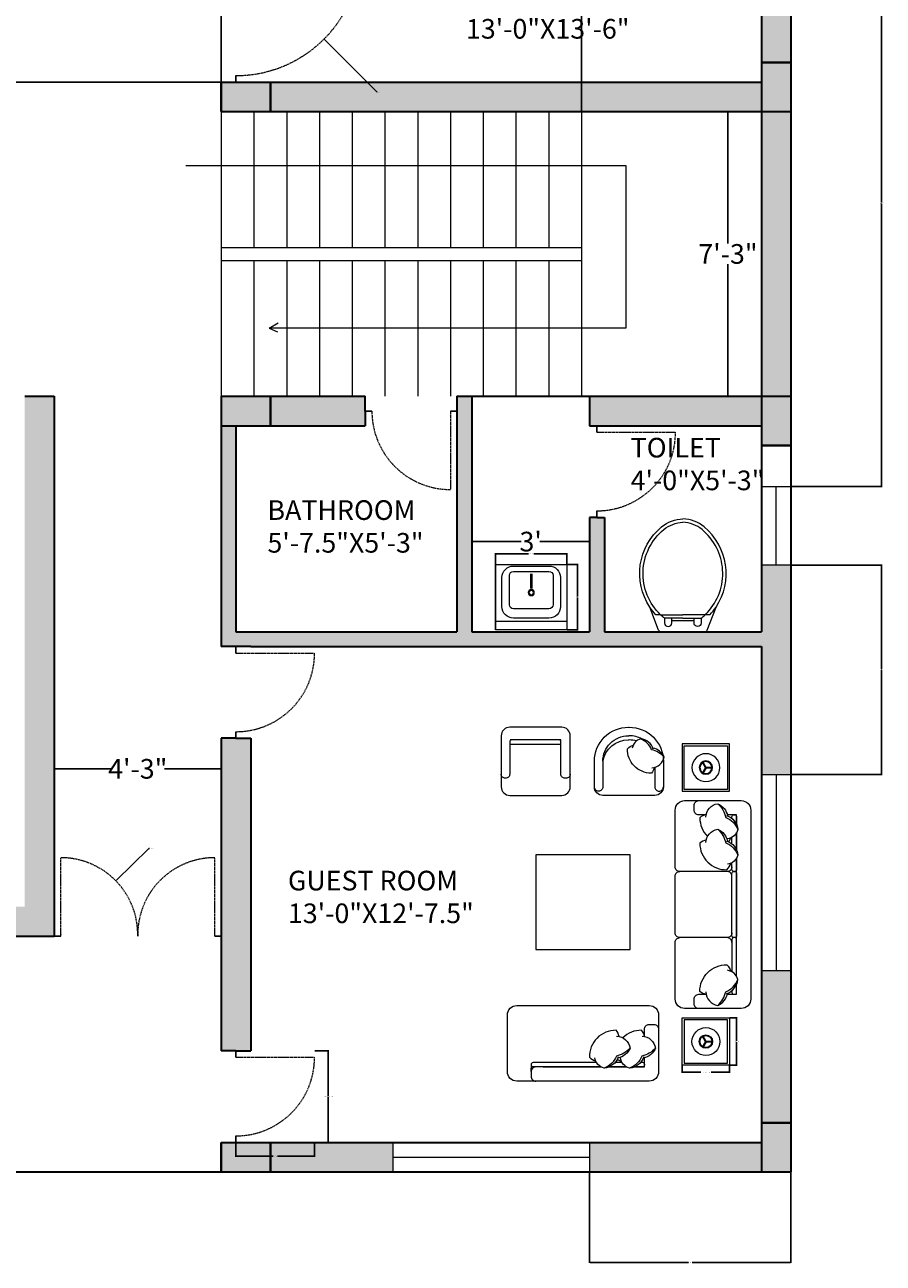
# Model space of a CAD drawing. Units: inches. Extents: x -10 to 455, y -513 to 57.
# Tile 2 of 4: x 193 to 455, y -513 to -134. Entities that reach past the tile are written whole.
import ezdxf

# ---------------------------------------------------------------- set-up
doc = ezdxf.new("R2010")
doc.units = ezdxf.units.IN
doc.header["$MEASUREMENT"] = 0
doc.linetypes.add('DASHED2', pattern=[0.375, 0.25, -0.125])
for name, color, linetype, lineweight in [('A-ANNO-DIMS', 2, 'Continuous', 18), ('A-AREA-IDEN', 7, 'Continuous', 18), ('A-COLS', 7, 'Continuous', 40), ('A-COLS-PATT', 1, 'Continuous', 13), ('A-DOOR', 40, 'DASHED2', 18), ('A-DOOR-FRAM', 7, 'Continuous', 25), ('A-FLOR-FIXT', 9, 'Continuous', 18), ('A-FLOR-STRS', 7, 'Continuous', 18), ('A-FURN', 8, 'Continuous', 13), ('A-GLAZ', 222, 'Continuous', 18), ('A-WALL', 7, 'Continuous', 35), ('A-WALL-PATT', 152, 'Continuous', 13)]:
    doc.layers.add(name, color=color, linetype=linetype, lineweight=lineweight)
doc.styles.get("Standard").update_dxf_attribs({"font": 'arial.ttf'})
doc.dimstyles.get("Standard").update_dxf_attribs({"dimtxt": 0.18, "dimasz": 0.18, "dimexe": 0.18, "dimexo": 0.0625, "dimgap": 0.09, "dimtad": 0, "dimtih": 1, "dimtoh": 1, "dimdec": 0, "dimzin": 0, "dimdsep": 46, "dimlunit": 3, "dimtxsty": 'Standard', "dimcen": 0.09, "dimadec": 0, "dimazin": 0, "dimtfac": 1, "dimtdec": 0, "dimtofl": 0, "dimtmove": 0, "dimatfit": 3, "dimfxl": 1, "dimtolj": 1, "dimtzin": 0, "dimarcsym": 0})

# ---------------------------------------------------------------- blocks, each defined once
blk = doc.blocks.new('*D3')
at = {"layer": 'A-ANNO-DIMS', "color": 0, "lineweight": -2, "transparency": 16777216}
for p, q in [((202.25, -359.95), (202.25, -361.87)), ((202.43, -361.69), (219.56, -361.69)), ((253.07, -361.69), (235.93, -361.69)), ((253.25, -359.95), (253.25, -361.87))]:
    blk.add_line(p, q, dxfattribs=at)
at = {"layer": 'A-ANNO-DIMS', "color": 0, "transparency": 16777216}
for points in [[(202.43, -361.66), (202.43, -361.72), (202.25, -361.69)], [(253.07, -361.66), (253.07, -361.72), (253.25, -361.69)]]:
    blk.add_solid(points, dxfattribs=at)
at = {"layer": 'Defpoints', "color": 0, "transparency": 16777216}
for p in [(202.25, -359.88), (202.25, -361.69), (253.25, -359.88)]:
    blk.add_point(p, dxfattribs=at)
at = {"layer": 'A-ANNO-DIMS', "color": 0, "transparency": 16777216, "insert": (227.75, -361.69), "char_height": 6, "attachment_point": 5}
blk.add_mtext('\\A1;4\'-3"', dxfattribs=at)
blk = doc.blocks.new('*D5')
at = {"layer": 'A-ANNO-DIMS', "color": 0, "lineweight": -2, "transparency": 16777216}
for p, q in [((406.12, -160.85), (408.18, -160.85)), ((408, -161.03), (408, -201.19)), ((408, -247.67), (408, -207.51)), ((406.12, -247.85), (408.18, -247.85))]:
    blk.add_line(p, q, dxfattribs=at)
at = {"layer": 'A-ANNO-DIMS', "color": 0, "transparency": 16777216}
for points in [[(407.97, -161.03), (408.03, -161.03), (408, -160.85)], [(407.97, -247.67), (408.03, -247.67), (408, -247.85)]]:
    blk.add_solid(points, dxfattribs=at)
at = {"layer": 'Defpoints', "color": 0, "transparency": 16777216}
for p in [(406.06, -160.85), (406.06, -247.85), (408, -247.85)]:
    blk.add_point(p, dxfattribs=at)
at = {"layer": 'A-ANNO-DIMS', "color": 0, "transparency": 16777216, "insert": (408, -204.35), "char_height": 6, "attachment_point": 5}
blk.add_mtext('\\A1;7\'-3"', dxfattribs=at)
blk = doc.blocks.new('*D6')
at = {"layer": 'A-ANNO-DIMS', "color": 0, "lineweight": -2, "transparency": 16777216}
for p, q in [((329.75, -291.29), (329.75, -292.44)), ((365.75, -291.29), (365.75, -292.44)), ((329.93, -292.26), (344.9, -292.26)), ((365.57, -292.26), (350.59, -292.26))]:
    blk.add_line(p, q, dxfattribs=at)
at = {"layer": 'A-ANNO-DIMS', "color": 0, "transparency": 16777216}
for points in [[(329.93, -292.23), (329.93, -292.29), (329.75, -292.26)], [(365.57, -292.23), (365.57, -292.29), (365.75, -292.26)]]:
    blk.add_solid(points, dxfattribs=at)
at = {"layer": 'Defpoints', "color": 0, "transparency": 16777216}
for p in [(329.75, -291.23), (365.75, -291.23), (365.75, -292.26)]:
    blk.add_point(p, dxfattribs=at)
at = {"layer": 'A-ANNO-DIMS', "color": 0, "transparency": 16777216, "insert": (347.75, -292.26), "char_height": 6, "attachment_point": 5}
blk.add_mtext("\\A1;3'", dxfattribs=at)
blk = doc.blocks.new('М14 600х655')
for p, q in [((-655, 600), (-655, 0)), ((-655, 600), (-655, 0)), ((-655, 0), (-655, 600)), ((0, 600), (-655, 600)), ((0, 0), (0, 600)), ((0, 525), (-655, 525)), ((-165, 494), (-490, 494)), ((-596, 388), (-596, 121)), ((-528, 370), (-528, 103)), ((-165, 408), (-490, 408)), ((-127, 103), (-127, 370)), ((-59, 121), (-59, 388)), ((-334, 87), (-334, 220)), ((-321, 87), (-321, 220)), ((-655, 0), (-655, 0)), ((-655, 0), (-655, 0)), ((-655, 0), (0, 0)), ((-655, 0), (0, 0)), ((-490, 65), (-165, 65)), ((-490, 15), (-165, 15))]:
    blk.add_line(p, q)
for radius in [27.6, 19.3]:
    blk.add_circle((-327, 259), radius)
for centre, radius, start, end in [((-490, 388), 106, 90, 180), ((-165, 388), 106, 0, 90), ((-490, 370), 38.2, 90, 180), ((-165, 370), 38.2, 0, 90), ((-490, 121), 106, 180, 270), ((-165, 121), 106, 270, 0), ((-490, 103), 38.2, 180, 270), ((-165, 103), 38.2, 270, 0)]:
    blk.add_arc(centre, radius, start, end)
blk = doc.blocks.new('WIN-60IN')
for p, q in [((0, 9), (60, 9)), ((0, 0), (0, 9)), ((60, 9), (60, 0)), ((0, 4.5), (60, 4.5)), ((60, 0), (0, 0))]:
    blk.add_line(p, q)
blk = doc.blocks.new('WIN-24IN')
for p, q in [((0, 9), (24, 9)), ((0, 0), (0, 9)), ((24, 9), (24, 0)), ((0, 4.5), (24, 4.5)), ((24, 0), (0, 0))]:
    blk.add_line(p, q)
blk = doc.blocks.new('DOOR-SINGLE-24IN')
for p, q in [((0, 28), (0, 26)), ((0, 26), (24, 26)), ((0, 0), (0, 2))]:
    blk.add_line(p, q)
blk.add_arc((0, 26), 24, 270, 0)
blk = doc.blocks.new('TABLE-END-WITH-LAMP')
for p, q in [((7.14, 7.17), (6.12, 8.93)), ((7.3, 7.26), (6.28, 9.03)), ((7.14, 7.26), (6.12, 5.5)), ((7.3, 7.17), (6.28, 5.41)), ((7.22, 7.31), (9.25, 7.31)), ((7.22, 7.13), (9.25, 7.13))]:
    blk.add_line(p, q)
at = {"ltscale": 0.03}
blk.add_lwpolyline([(0, 0), (0, 14.43), (14.43, 14.43), (14.43, 0)], close=True, dxfattribs=at)
blk.add_lwpolyline([(0.58, 13.86), (0.58, 0.58), (13.86, 0.58), (13.86, 13.86)], close=True)
for radius in [4.26, 2.04, 1.83]:
    blk.add_circle((7.22, 7.22), radius)
blk = doc.blocks.new('*D16')
at = {"layer": 'A-ANNO-DIMS', "color": 0, "lineweight": -2, "transparency": 16777216}
for p, q in [((281.81, -447.85), (286.13, -447.85)), ((285.95, -448.03), (285.95, -461.67)), ((285.95, -475.67), (285.95, -462.03)), ((281.81, -475.85), (286.13, -475.85))]:
    blk.add_line(p, q, dxfattribs=at)
at = {"layer": 'A-ANNO-DIMS', "color": 0, "transparency": 16777216}
for points in [[(285.92, -448.03), (285.98, -448.03), (285.95, -447.85)], [(285.92, -475.67), (285.98, -475.67), (285.95, -475.85)]]:
    blk.add_solid(points, dxfattribs=at)
at = {"layer": 'Defpoints', "color": 0, "transparency": 16777216}
for p in [(281.75, -447.85), (285.95, -447.85), (281.75, -475.85)]:
    blk.add_point(p, dxfattribs=at)
at = {"layer": 'A-ANNO-DIMS', "color": 0, "transparency": 16777216, "insert": (285.95, -461.85), "char_height": 0.18, "attachment_point": 5}
blk.add_mtext('\\A1;SINGLE DOOR 2\'-4" TYP.', dxfattribs=at)
blk = doc.blocks.new('*D17')
at = {"layer": 'A-ANNO-DIMS', "color": 0, "lineweight": -2, "transparency": 16777216}
for p, q in [((257.75, -475.91), (257.75, -480.23)), ((281.75, -475.91), (281.75, -480.23)), ((257.93, -480.05), (269.11, -480.05)), ((281.57, -480.05), (270.39, -480.05))]:
    blk.add_line(p, q, dxfattribs=at)
at = {"layer": 'A-ANNO-DIMS', "color": 0, "transparency": 16777216}
for points in [[(257.93, -480.02), (257.93, -480.08), (257.75, -480.05)], [(281.57, -480.02), (281.57, -480.08), (281.75, -480.05)]]:
    blk.add_solid(points, dxfattribs=at)
at = {"layer": 'Defpoints', "color": 0, "transparency": 16777216}
for p in [(257.75, -475.85), (281.75, -475.85), (281.75, -480.05)]:
    blk.add_point(p, dxfattribs=at)
at = {"layer": 'A-ANNO-DIMS', "color": 0, "transparency": 16777216, "insert": (269.75, -480.05), "char_height": 0.18, "attachment_point": 5}
blk.add_mtext('\\A1;2\'-0" TYP.', dxfattribs=at)
blk = doc.blocks.new('*D20')
at = {"layer": 'A-ANNO-DIMS', "color": 0, "lineweight": -2, "transparency": 16777216}
for p, q in [((337.03, -299.16), (337.03, -295.77)), ((337.21, -295.95), (347.11, -295.95)), ((358.64, -295.95), (348.73, -295.95)), ((358.82, -299.16), (358.82, -295.77))]:
    blk.add_line(p, q, dxfattribs=at)
at = {"layer": 'A-ANNO-DIMS', "color": 0, "transparency": 16777216}
for points in [[(337.21, -295.92), (337.21, -295.98), (337.03, -295.95)], [(358.64, -295.92), (358.64, -295.98), (358.82, -295.95)]]:
    blk.add_solid(points, dxfattribs=at)
at = {"layer": 'Defpoints', "color": 0, "transparency": 16777216}
for p in [(358.82, -295.95), (337.03, -299.22), (358.82, -299.22)]:
    blk.add_point(p, dxfattribs=at)
at = {"layer": 'A-ANNO-DIMS', "color": 0, "transparency": 16777216, "insert": (347.92, -295.95), "char_height": 0.18, "attachment_point": 5}
blk.add_mtext('\\A1;BASIN 1\'-10"', dxfattribs=at)
blk = doc.blocks.new('*D21')
at = {"layer": 'A-ANNO-DIMS', "color": 0, "lineweight": -2, "transparency": 16777216}
for p, q in [((358.88, -299.22), (362.26, -299.22)), ((362.08, -299.4), (362.08, -309.02)), ((362.08, -319), (362.08, -309.38)), ((358.88, -319.18), (362.26, -319.18))]:
    blk.add_line(p, q, dxfattribs=at)
at = {"layer": 'A-ANNO-DIMS', "color": 0, "transparency": 16777216}
for points in [[(362.05, -299.4), (362.11, -299.4), (362.08, -299.22)], [(362.05, -319), (362.11, -319), (362.08, -319.18)]]:
    blk.add_solid(points, dxfattribs=at)
at = {"layer": 'Defpoints', "color": 0, "transparency": 16777216}
for p in [(358.82, -299.22), (358.82, -319.18), (362.08, -319.18)]:
    blk.add_point(p, dxfattribs=at)
at = {"layer": 'A-ANNO-DIMS', "color": 0, "transparency": 16777216, "insert": (362.08, -309.2), "char_height": 0.18, "attachment_point": 5}
blk.add_mtext('\\A1;1\'-8"', dxfattribs=at)
blk = doc.blocks.new('*D24')
at = {"layer": 'A-ANNO-DIMS', "color": 0, "lineweight": -2, "transparency": 16777216}
for p, q in [((394.05, -452.31), (394.05, -454.6)), ((408.48, -452.31), (408.48, -454.6)), ((394.23, -454.42), (399.69, -454.42)), ((408.3, -454.42), (402.84, -454.42))]:
    blk.add_line(p, q, dxfattribs=at)
at = {"layer": 'A-ANNO-DIMS', "color": 0, "transparency": 16777216}
for points in [[(394.23, -454.39), (394.23, -454.45), (394.05, -454.42)], [(408.3, -454.39), (408.3, -454.45), (408.48, -454.42)]]:
    blk.add_solid(points, dxfattribs=at)
at = {"layer": 'Defpoints', "color": 0, "transparency": 16777216}
for p in [(394.05, -452.25), (408.48, -452.25), (408.48, -454.42)]:
    blk.add_point(p, dxfattribs=at)
at = {"layer": 'A-ANNO-DIMS', "color": 0, "transparency": 16777216, "insert": (401.26, -454.42), "char_height": 0.18, "attachment_point": 5}
blk.add_mtext('\\A1;END TABLE 1\'-2 1/2" TYP.', dxfattribs=at)
blk = doc.blocks.new('*D25')
at = {"layer": 'A-ANNO-DIMS', "color": 0, "lineweight": -2, "transparency": 16777216}
for p, q in [((408.54, -437.82), (410.83, -437.82)), ((410.65, -438), (410.65, -444.85)), ((410.65, -452.07), (410.65, -445.22)), ((408.54, -452.25), (410.83, -452.25))]:
    blk.add_line(p, q, dxfattribs=at)
at = {"layer": 'A-ANNO-DIMS', "color": 0, "transparency": 16777216}
for points in [[(410.62, -438), (410.68, -438), (410.65, -437.82)], [(410.62, -452.07), (410.68, -452.07), (410.65, -452.25)]]:
    blk.add_solid(points, dxfattribs=at)
at = {"layer": 'Defpoints', "color": 0, "transparency": 16777216}
for p in [(408.48, -437.82), (410.65, -437.82), (408.48, -452.25)]:
    blk.add_point(p, dxfattribs=at)
at = {"layer": 'A-ANNO-DIMS', "color": 0, "transparency": 16777216, "insert": (410.65, -445.03), "char_height": 0.18, "attachment_point": 5}
blk.add_mtext('\\A1;1\'-2 1/2" TYP.', dxfattribs=at)
blk = doc.blocks.new('*D38')
at = {"layer": 'A-ANNO-DIMS', "color": 0, "lineweight": -2, "transparency": 16777216}
for p, q in [((427.31, -102.17), (455.08, -102.17)), ((454.9, -102.35), (454.9, -188.62)), ((454.9, -275.26), (454.9, -188.98)), ((427.31, -275.44), (455.08, -275.44))]:
    blk.add_line(p, q, dxfattribs=at)
at = {"layer": 'A-ANNO-DIMS', "color": 0, "transparency": 16777216}
for points in [[(454.87, -102.35), (454.93, -102.35), (454.9, -102.17)], [(454.87, -275.26), (454.93, -275.26), (454.9, -275.44)]]:
    blk.add_solid(points, dxfattribs=at)
at = {"layer": 'Defpoints', "color": 0, "transparency": 16777216}
for p in [(427.25, -102.17), (427.25, -275.44), (454.9, -275.44)]:
    blk.add_point(p, dxfattribs=at)
at = {"layer": 'A-ANNO-DIMS', "color": 0, "transparency": 16777216, "insert": (454.9, -188.8), "char_height": 0.18, "attachment_point": 5}
blk.add_mtext('\\A1;14\'-5 1/2"', dxfattribs=at)
blk = doc.blocks.new('*D39')
at = {"layer": 'A-ANNO-DIMS', "color": 0, "lineweight": -2, "transparency": 16777216}
for p, q in [((427.31, -299.44), (455.08, -299.44)), ((454.9, -299.62), (454.9, -331.23)), ((454.9, -363.21), (454.9, -331.59)), ((427.31, -363.39), (455.08, -363.39))]:
    blk.add_line(p, q, dxfattribs=at)
at = {"layer": 'A-ANNO-DIMS', "color": 0, "transparency": 16777216}
for points in [[(454.87, -299.62), (454.93, -299.62), (454.9, -299.44)], [(454.87, -363.21), (454.93, -363.21), (454.9, -363.39)]]:
    blk.add_solid(points, dxfattribs=at)
at = {"layer": 'Defpoints', "color": 0, "transparency": 16777216}
for p in [(427.25, -299.44), (427.25, -363.39), (454.9, -363.39)]:
    blk.add_point(p, dxfattribs=at)
at = {"layer": 'A-ANNO-DIMS', "color": 0, "transparency": 16777216, "insert": (454.9, -331.41), "char_height": 0.18, "attachment_point": 5}
blk.add_mtext('\\A1;5\'-4"', dxfattribs=at)
blk = doc.blocks.new('*D40')
at = {"layer": 'A-ANNO-DIMS', "color": 0, "lineweight": -2, "transparency": 16777216}
for p, q in [((365.75, -484.91), (365.75, -512.68)), ((427.25, -484.91), (427.25, -512.68)), ((365.93, -512.5), (395.96, -512.5)), ((427.07, -512.5), (397.04, -512.5))]:
    blk.add_line(p, q, dxfattribs=at)
at = {"layer": 'A-ANNO-DIMS', "color": 0, "transparency": 16777216}
for points in [[(365.93, -512.47), (365.93, -512.53), (365.75, -512.5)], [(427.07, -512.47), (427.07, -512.53), (427.25, -512.5)]]:
    blk.add_solid(points, dxfattribs=at)
at = {"layer": 'Defpoints', "color": 0, "transparency": 16777216}
for p in [(365.75, -484.85), (427.25, -484.85), (427.25, -512.5)]:
    blk.add_point(p, dxfattribs=at)
at = {"layer": 'A-ANNO-DIMS', "color": 0, "transparency": 16777216, "insert": (396.5, -512.5), "char_height": 0.18, "attachment_point": 5}
blk.add_mtext('\\A1;5\'-1 1/2"', dxfattribs=at)
blk = doc.blocks.new('*D41')
at = {"layer": 'A-ANNO-DIMS', "color": 0, "lineweight": -2, "transparency": 16777216}
for p, q in [((253.25, -160.79), (253.25, 46.98)), ((253.43, 46.8), (307.92, 46.8)), ((363.07, 46.8), (308.58, 46.8)), ((363.25, -160.79), (363.25, 46.98))]:
    blk.add_line(p, q, dxfattribs=at)
at = {"layer": 'A-ANNO-DIMS', "color": 0, "transparency": 16777216}
for points in [[(253.43, 46.83), (253.43, 46.77), (253.25, 46.8)], [(363.07, 46.83), (363.07, 46.77), (363.25, 46.8)]]:
    blk.add_solid(points, dxfattribs=at)
at = {"layer": 'Defpoints', "color": 0, "transparency": 16777216}
for p in [(363.25, 46.8), (253.25, -160.85), (363.25, -160.85)]:
    blk.add_point(p, dxfattribs=at)
at = {"layer": 'A-ANNO-DIMS', "color": 0, "transparency": 16777216, "insert": (308.25, 46.8), "char_height": 0.18, "attachment_point": 5}
blk.add_mtext('\\A1;9\'-2"', dxfattribs=at)
blk = doc.blocks.new('*D43')
at = {"layer": 'A-ANNO-DIMS', "color": 0, "lineweight": -2, "transparency": 16777216}
for p, q in [((253.18, -109.85), (12.42, -109.85)), ((12.6, -110.03), (12.6, -130.67)), ((12.6, -151.67), (12.6, -131.03)), ((253.18, -151.85), (12.42, -151.85))]:
    blk.add_line(p, q, dxfattribs=at)
at = {"layer": 'A-ANNO-DIMS', "color": 0, "transparency": 16777216}
for points in [[(12.57, -110.03), (12.63, -110.03), (12.6, -109.85)], [(12.57, -151.67), (12.63, -151.67), (12.6, -151.85)]]:
    blk.add_solid(points, dxfattribs=at)
at = {"layer": 'Defpoints', "color": 0, "transparency": 16777216}
for p in [(253.25, -109.85), (12.6, -151.85), (253.25, -151.85)]:
    blk.add_point(p, dxfattribs=at)
at = {"layer": 'A-ANNO-DIMS', "color": 0, "transparency": 16777216, "insert": (12.6, -130.85), "char_height": 0.18, "attachment_point": 5}
blk.add_mtext('\\A1;3\'-6"', dxfattribs=at)
blk = doc.blocks.new('*D45')
at = {"layer": 'A-ANNO-DIMS', "color": 0, "lineweight": -2, "transparency": 16777216}
for p, q in [((257.66, -111.85), (257.84, -111.85)), ((257.75, -111.94), (257.75, -111.76)), ((300.74, -154.84), (284.74, -138.85)), ((300.92, -154.84), (300.74, -154.84))]:
    blk.add_line(p, q, dxfattribs=at)
at = {"layer": 'A-ANNO-DIMS', "color": 0, "transparency": 16777216}
blk.add_solid([(284.76, -138.83), (284.72, -138.87), (284.62, -138.72)], dxfattribs=at)
at = {"layer": 'Defpoints', "color": 0, "transparency": 16777216}
for p in [(257.75, -111.85), (284.62, -138.72)]:
    blk.add_point(p, dxfattribs=at)
at = {"layer": 'A-ANNO-DIMS', "color": 0, "transparency": 16777216, "insert": (301.33, -154.84), "char_height": 0.18, "attachment_point": 5}
blk.add_mtext('\\A1;R3\'-2"', dxfattribs=at)
blk = doc.blocks.new('*D46')
at = {"layer": 'A-ANNO-DIMS', "color": 0, "lineweight": -2, "transparency": 16777216}
for p, q in [((231.12, -386.04), (221.17, -395.79)), ((231.3, -386.04), (231.12, -386.04)), ((204.16, -412.36), (204.34, -412.36)), ((204.25, -412.45), (204.25, -412.27))]:
    blk.add_line(p, q, dxfattribs=at)
at = {"layer": 'A-ANNO-DIMS', "color": 0, "transparency": 16777216}
blk.add_solid([(221.15, -395.76), (221.19, -395.81), (221.04, -395.91)], dxfattribs=at)
at = {"layer": 'Defpoints', "color": 0, "transparency": 16777216}
for p in [(221.04, -395.91), (204.25, -412.36)]:
    blk.add_point(p, dxfattribs=at)
at = {"layer": 'A-ANNO-DIMS', "color": 0, "transparency": 16777216, "insert": (232.19, -386.04), "char_height": 0.18, "attachment_point": 5}
blk.add_mtext('\\A1;2X R1\'-11 1/2"', dxfattribs=at)

msp = doc.modelspace()

# ---------------------------------------------------------------- hatches: boundary and pattern name
at = {"layer": 'A-COLS-PATT'}
h = msp.add_hatch(color=256, dxfattribs=at)
h.dxf.hatch_style = 1
h.paths.add_polyline_path([(55.25, 19.15), (40.25, 19.15), (40.25, 10.15), (55.25, 10.15)])
h.paths.add_polyline_path([(262.25, 19.15), (253.25, 19.15), (253.25, 4.15), (262.25, 4.15)])
h.paths.add_polyline_path([(427.25, 19.15), (418.25, 19.15), (418.25, 4.15), (427.25, 4.15)])
h.paths.add_polyline_path([(427.25, -247.85), (418.25, -247.85), (418.25, -262.85), (427.25, -262.85)])
h.paths.add_polyline_path([(268.25, -247.85), (253.25, -247.85), (253.25, -256.85), (268.25, -256.85)])
h.paths.add_polyline_path([(55.25, -247.85), (40.25, -247.85), (40.25, -256.85), (55.25, -256.85)])
h.paths.add_polyline_path([(55.25, -475.85), (49.25, -475.85), (40.25, -475.85), (40.25, -484.85), (55.25, -484.85)])
h.paths.add_polyline_path([(268.25, -475.85), (253.25, -475.85), (253.25, -484.85), (268.25, -484.85)])
h.paths.add_polyline_path([(427.25, -469.85), (418.25, -469.85), (418.25, -484.85), (427.25, -484.85)])
h.paths.add_polyline_path([(55.25, -100.85), (40.25, -100.85), (40.25, -109.85), (55.25, -109.85)])
h = msp.add_hatch(color=256, dxfattribs=at)
h.dxf.hatch_style = 1
h.paths.add_polyline_path([(268.25, -151.85), (253.25, -151.85), (253.25, -160.85), (268.25, -160.85)])
h.paths.add_polyline_path([(427.25, -145.85), (418.25, -145.85), (418.25, -160.85), (427.25, -160.85)])
at = {"layer": 'A-WALL-PATT'}
h = msp.add_hatch(color=256, dxfattribs=at)
h.dxf.hatch_style = 1
h.paths.add_polyline_path([(418.25, -151.85), (268.25, -151.85), (268.25, -160.85), (418.25, -160.85)])
h.paths.add_polyline_path([(165.25, -100.85), (55.25, -100.85), (55.25, -109.85), (165.25, -109.85), (165.25, -105.35)])
h.paths.add_polyline_path([(49.25, -75.35), (40.25, -75.35), (40.25, -100.85), (49.25, -100.85)])
h.paths.add_polyline_path([(49.25, 10.15), (40.25, 10.15), (40.25, -15.35), (49.25, -15.35)])
h.paths.add_polyline_path([(86.75, 19.15), (55.25, 19.15), (55.25, 10.15), (86.75, 10.15)])
h.paths.add_polyline_path([(213.5, 19.15), (146.75, 19.15), (146.75, 10.15), (193.25, 10.15), (193.25, -28.04), (197.75, -28.04), (197.75, 10.15), (213.5, 10.15)])
h.paths.add_polyline_path([(262.25, 4.15), (253.25, 4.15), (253.25, -69.35), (197.75, -69.35), (197.75, -60), (193.25, -60), (193.25, -109.85), (197.75, -109.85), (197.75, -73.85), (253.25, -73.85), (253.25, -109.85), (262.25, -109.85)])
h.paths.add_polyline_path([(310.25, 19.15), (262.25, 19.15), (262.25, 10.15), (310.25, 10.15)])
h.paths.add_polyline_path([(253.25, 19.15), (237.5, 19.15), (237.5, 10.15), (253.25, 10.15)])
h.paths.add_polyline_path([(418.25, 19.15), (370.25, 19.15), (370.25, 10.15), (418.25, 10.15)])
h.paths.add_polyline_path([(427.25, 4.15), (418.25, 4.15), (418.25, -42.17), (427.25, -42.17)])
h.paths.add_polyline_path([(427.25, -102.17), (418.25, -102.17), (418.25, -145.85), (427.25, -145.85)])
h.paths.add_polyline_path([(427.25, -160.85), (418.25, -160.85), (418.25, -247.85), (427.25, -247.85)])
h.paths.add_polyline_path([(418.25, -247.85), (365.75, -247.85), (365.75, -256.85), (418.25, -256.85)], flags=17)
h.paths.add_polyline_path([(297.25, -247.85), (268.25, -247.85), (268.25, -256.85), (297.25, -256.85), (297.25, -252.35)], flags=17)
h.paths.add_polyline_path([(427.25, -299.44), (418.25, -299.44), (418.25, -319.85), (370.25, -319.85), (370.25, -284.85), (368, -284.85), (365.75, -284.85), (365.75, -319.85), (329.75, -319.85), (329.75, -247.85), (325.25, -247.85), (325.25, -319.85), (257.75, -319.85), (257.75, -256.85), (253.25, -256.85), (253.25, -324.35), (262.25, -324.35), (418.25, -324.35), (418.25, -363.39), (427.25, -363.39)])
h.paths.add_polyline_path([(262.25, -352.35), (257.75, -352.35), (253.25, -352.35), (253.25, -447.85), (257.75, -447.85), (262.25, -447.85)])
h.paths.add_polyline_path([(305.75, -475.85), (268.25, -475.85), (268.25, -484.85), (305.75, -484.85)])
h.paths.add_polyline_path([(418.25, -475.85), (365.75, -475.85), (365.75, -484.85), (418.25, -484.85)])
h.paths.add_polyline_path([(427.25, -423.39), (418.25, -423.39), (418.25, -469.85), (427.25, -469.85)])
h.paths.add_polyline_path([(202.25, -247.85), (193.25, -247.85), (193.25, -403.85), (49.25, -403.85), (49.25, -360.35), (40.25, -360.35), (40.25, -412.85), (202.25, -412.85)])
h.paths.add_polyline_path([(165.25, -247.85), (55.25, -247.85), (55.25, -256.85), (165.25, -256.85), (165.25, -252.35)], flags=17)
h.paths.add_polyline_path([(49.25, -225.11), (40.25, -225.11), (40.25, -247.85), (49.25, -247.85)])
h.paths.add_polyline_path([(49.25, -256.85), (40.25, -256.85), (40.25, -300.35), (49.25, -300.35)], flags=17)
h.paths.add_polyline_path([(49.25, -137.85), (44.75, -137.85), (40.25, -137.85), (40.25, -165.11), (49.25, -165.11)])

# ---------------------------------------------------------------- linework, layer by layer
at = {"layer": 'A-COLS'}
for p, q in [((418.25, -145.85), (427.25, -145.85)), ((253.25, -151.85), (253.25, -160.85)), ((268.25, -151.85), (268.25, -160.85)), ((268.25, -256.85), (268.25, -247.85)), ((418.25, -262.85), (427.25, -262.85)), ((418.25, -469.85), (427.25, -469.85)), ((253.25, -475.85), (253.25, -484.85)), ((268.25, -475.85), (268.25, -484.85))]:
    msp.add_line(p, q, dxfattribs=at)
at = {"layer": 'A-DOOR'}
for p, q in [((257.75, -149.85), (257.75, -151.85)), ((204.25, -412.85), (204.25, -388.85)), ((251.25, -412.85), (251.25, -388.85)), ((202.25, -412.85), (204.25, -412.85)), ((253.25, -412.85), (251.25, -412.85))]:
    msp.add_line(p, q, dxfattribs=at)
for centre, radius, start, end in [((257.75, -111.85), 38, 270, 0), ((204.25, -412.36), 23.51, 358.7938, 90), ((251.25, -412.36), 23.51, 90, 181.2062)]:
    msp.add_arc(centre, radius, start, end, dxfattribs=at)
at = {"layer": 'A-DOOR-FRAM'}
for p, q in [((257.75, -151.85), (257.75, -149.85)), ((299.25, -252.35), (297.25, -252.35)), ((325.25, -252.35), (323.25, -252.35)), ((368, -256.85), (368, -258.85)), ((368, -282.85), (368, -284.85)), ((257.75, -324.35), (257.75, -326.35)), ((257.75, -350.35), (257.75, -352.35)), ((202.25, -412.85), (204.25, -412.85)), ((253.25, -412.85), (251.25, -412.85)), ((257.75, -449.85), (257.75, -447.85)), ((257.75, -475.85), (257.75, -473.85))]:
    msp.add_line(p, q, dxfattribs=at)
at = {"layer": 'A-FLOR-FIXT'}
for p, q in [((387.45, -314.62), (386, -314.62)), ((387.45, -314.62), (394.25, -314.62)), ((401.04, -314.62), (394.25, -314.62)), ((402.49, -314.62), (401.04, -314.62))]:
    msp.add_line(p, q, dxfattribs=at)
for points in [[(384.13, -312.25, -0.383919), (387.75, -287.78, -0.163732), (394.25, -285.29, -0.359733)], [(387.45, -314.62, -0.448546), (388.41, -288.58, -0.162618), (394.25, -286.33, -0.470877)], [(404.36, -312.25, 0.383919), (400.74, -287.78, 0.163732), (394.25, -285.29, 0.359733)], [(401.74, -313.91, 0.431639), (400.08, -288.58, 0.162618), (394.25, -286.33, 0.470877)], [(386, -314.62, -0.040937), (384.13, -312.25, -0.163732)], [(394.25, -319.85), (387.65, -319.85, -0.31031), (386.84, -319.3), (384.13, -312.25, -0.209071)], [(394.25, -319.85), (400.84, -319.85, 0.31031), (401.65, -319.3), (404.36, -312.25, 0.209071)], [(401.04, -314.62, 0.014165), (401.74, -313.91, 0.162618)], [(402.49, -314.62, 0.040937), (404.36, -312.25, 0.163732)], [(388.64, -315.66, -0.022712), (387.45, -314.62, -0.162618)], [(394.25, -315.66), (388.64, -315.66, -0.476108)], [(388.64, -315.66), (388.64, -317.11, 1), (390.84, -317.11), (390.84, -316.36)], [(394.25, -315.66), (399.85, -315.66, 0.022712)], [(399.85, -315.66), (399.85, -317.11, -1), (397.65, -317.11), (397.65, -316.36)], [(399.85, -315.66, 0.022712), (401.04, -314.62, 0.162618)]]:
    msp.add_lwpolyline(points, format="xyb", dxfattribs=at)
for points in [[(390.84, -316.36), (390.84, -315.66)], [(390.84, -316.36), (397.65, -316.36)], [(397.65, -316.36), (397.65, -315.66)]]:
    msp.add_lwpolyline(points, dxfattribs=at)
at = {"layer": 'A-FLOR-STRS'}
for p, q in [((253.25, -160.85), (253.25, -247.85)), ((263.25, -160.85), (263.25, -202.35)), ((273.25, -160.85), (273.25, -202.35)), ((283.25, -160.85), (283.25, -202.35)), ((293.25, -160.85), (293.25, -202.35)), ((303.25, -160.85), (303.25, -202.35)), ((313.25, -160.85), (313.25, -202.35)), ((323.25, -160.85), (323.25, -202.35)), ((333.25, -160.85), (333.25, -202.35)), ((343.25, -160.85), (343.25, -202.35)), ((353.25, -160.85), (353.25, -202.35)), ((363.25, -160.85), (363.25, -247.85)), ((242.44, -177.35), (376.77, -177.35)), ((376.77, -177.35), (376.77, -227.04)), ((253.25, -202.35), (363.25, -202.35)), ((253.25, -206.35), (363.25, -206.35)), ((263.25, -206.35), (263.25, -247.85)), ((273.25, -206.35), (273.25, -247.85)), ((283.25, -206.35), (283.25, -247.85)), ((293.25, -206.35), (293.25, -247.85)), ((303.25, -206.35), (303.25, -247.85)), ((313.25, -206.35), (313.25, -247.85)), ((323.25, -206.35), (323.25, -247.85)), ((333.25, -206.35), (333.25, -247.85)), ((343.25, -206.35), (343.25, -247.85)), ((353.25, -206.35), (353.25, -247.85)), ((267.87, -227.04), (270.59, -225.4)), ((376.77, -227.04), (267.87, -227.04)), ((267.87, -227.04), (270.38, -228.11))]:
    msp.add_line(p, q, dxfattribs=at)
at = {"layer": 'A-FURN'}
msp.add_line((347.86, -454.23), (348, -452.07), dxfattribs=at)
at = {"layer": 'A-FURN', "ltscale": 0.03}
for points in [[(341.36, -348.98), (341.36, -348.98, 0.414214), (338.75, -351.58), (338.75, -367.2, 0.414214), (341.36, -369.8), (341.36, -369.8), (357.23, -369.8, 0.414214), (359.84, -367.2), (359.84, -351.58, 0.414214), (357.23, -348.98)], [(394.77, -434.93, -0.414214), (391.88, -432.04), (391.88, -414.72, -0.414214), (393.33, -413.28, -0.414214), (391.88, -411.83), (391.88, -394.51, -0.414214), (393.33, -393.07, -0.414214), (391.88, -391.63), (391.88, -374.31, -0.414214), (394.77, -371.42), (412.09, -371.42, -0.414214), (414.98, -374.31), (414.98, -432.04, -0.414214), (412.09, -434.93)], [(340.64, -436.91, -0.414214), (343.53, -434.02), (343.53, -434.02, 0.317837), (343.53, -434.02, -0.414214), (343.53, -434.02), (343.53, -434.02, 1.186185), (343.53, -434.02, -0.414214), (343.53, -434.02), (383.94, -434.02, -0.414214), (386.83, -436.91), (386.83, -454.23, -0.414214), (383.94, -457.12), (343.53, -457.12, -0.414214), (340.64, -454.23)]]:
    msp.add_lwpolyline(points, format="xyb", close=True, dxfattribs=at)
msp.add_lwpolyline([(377.74, -369.8), (369.8, -369.8, -0.414214), (367.2, -367.2), (367.2, -359.39, -0.414214), (377.61, -348.98), (377.74, -348.98), (377.87, -348.98, -0.414214), (388.28, -359.39), (388.28, -367.2, -0.414214), (385.68, -369.8), (377.74, -369.8)], format="xyb", dxfattribs=at)
at = {"layer": 'A-FURN'}
for points in [[(369.8, -359.39, -0.414214), (377.61, -351.58), (377.74, -351.58)], [(381.74, -352.61, 0.130591), (377.87, -351.58), (377.74, -351.58)], [(341.36, -353.66), (341.36, -363.29, -0.414214), (340.05, -364.59), (340.05, -364.59, -0.414214), (338.75, -363.29)], [(352.07, -352.88), (341.88, -352.88, 0.414214), (341.36, -353.4), (341.36, -353.66, 0.414214), (341.88, -354.18), (350.76, -354.18, 0.414214)], [(350.76, -354.18), (356.45, -354.18, 0.414214), (356.97, -353.66), (356.97, -353.4, 0.414214), (356.45, -352.88)], [(356.45, -352.88), (352.07, -352.88, 0.414214)], [(369.8, -359.39, -0.372719), (377.61, -352.88), (377.74, -352.88)], [(385.42, -361.28, -0.165541), (384.61, -363, -0.425989), (377.3, -355.54, -0.121523), (379.04, -354.51, 7.115464)], [(380.09, -353.16, 0.072384), (377.87, -352.88), (377.74, -352.88)], [(385.21, -355.66, 0.306663), (381.33, -352.56, 0.30633), (378.8, -355.39, -0.872847)], [(388.49, -358.07, 0.14773), (384.69, -355.84, 0.213343), (381.33, -352.56, 0.178662)], [(384.76, -361.35, 0.356772), (388.49, -358.07, 0.249542), (385.11, -355.37, -9.61688)], [(369.8, -359.39), (369.8, -367.2, -0.414214), (368.5, -368.5), (368.5, -368.5, -0.414214), (367.2, -367.2)], [(359.84, -363.29, -0.414214), (358.54, -364.59), (358.28, -364.59, -0.414214), (356.97, -363.29), (356.97, -361.28)], [(385.68, -361.21), (385.68, -367.2, 0.414214), (386.98, -368.5), (386.98, -368.5, 0.414214), (388.28, -367.2)], [(401.34, -375.75), (399.1, -375.75, -0.414214), (397.66, -374.31), (397.66, -372.86, -0.414214), (399.1, -371.42)], [(401.25, -376.47, -0.356772), (404.89, -372.34, -0.249542), (407.89, -376.08)], [(404.89, -372.34, -0.14773), (407.37, -376.56, -0.213343), (411.01, -380.28)], [(401.34, -375.75, 0.165541), (399.43, -376.64, 0.200231), (401.75, -382.37)], [(407.57, -375.97, -0.306663), (411.01, -380.28, -0.30633), (407.86, -383.09)], [(410.65, -378.79), (410.65, -375.75), (407.81, -375.75, -0.414352)], [(409.2, -376.85), (409.2, -376.33, -0.414214), (409.78, -375.75), (410.07, -375.75, -0.414214), (410.65, -376.33)], [(410.65, -376.33), (410.65, -378.79, -0.414469)], [(401.25, -384.25, -0.356772), (404.89, -380.11, -0.249542), (407.89, -383.86)], [(404.89, -380.11, -0.14773), (407.37, -384.33, -0.213343), (411.01, -388.05)], [(410.65, -381.19), (410.65, -386.56, -0.414747)], [(401.34, -383.52, 0.165541), (399.43, -384.41, 0.425989), (407.7, -392.52, 0.121523), (408.84, -390.6)], [(407.57, -383.75, -0.306663), (411.01, -388.05, -0.30633), (407.86, -390.87)], [(408.27, -384.03, 0.071865), (408.84, -382.82)], [(409.2, -384.63), (409.2, -382.64, -0.414599)], [(410.65, -388.96), (410.65, -392.49, -0.414214), (410.07, -393.07), (409.78, -393.07, -0.414214), (409.2, -392.49), (409.2, -390.42, -0.126313)], [(409.2, -391.63, -0.414214), (407.76, -393.07), (393.33, -393.07, -0.41732)], [(409.2, -394.51, 0.414214), (407.76, -393.07)], [(409.2, -411.83, -0.414214), (407.76, -413.28)], [(409.2, -414.72, 0.414214), (407.76, -413.28), (393.33, -413.28, 0.415249)], [(410.65, -425.16), (410.65, -413.86, 0.414214), (410.07, -413.28), (409.78, -413.28, 0.414214), (409.2, -413.86), (409.2, -423.71, 0.412652)], [(401.34, -430.6, -0.165541), (399.43, -429.71, -0.425989), (407.7, -421.6, -0.121523), (408.84, -423.53)], [(407.57, -430.37, 0.306663), (411.01, -426.07, 0.30633), (407.86, -423.26)], [(404.89, -434.01, 0.14773), (407.37, -429.79, 0.213343), (411.01, -426.07)], [(410.65, -430.02), (410.65, -427.56, 0.412535)], [(399.1, -434.93, -0.414214), (397.66, -433.49), (397.66, -432.04, -0.414214), (399.1, -430.6), (401.34, -430.6)], [(401.25, -429.87, 0.356772), (404.89, -434.01, 0.249542), (407.89, -430.26)], [(409.2, -429.5), (409.2, -430.02, 0.414214), (409.78, -430.6), (410.07, -430.6, 0.414214), (410.65, -430.02)], [(374.73, -443.48, 0.165541), (373.83, -441.57, 0.425989), (365.73, -449.84, 0.121523), (367.65, -450.98, -7.115464)], [(382.5, -443.48, 0.165541), (381.61, -441.57, 0.200231), (375.88, -443.89, 0.121523)], [(382.5, -443.48), (382.5, -441.24, -0.414214), (383.94, -439.8), (385.39, -439.8, -0.414214), (386.83, -441.24)], [(374, -443.39, -0.356772), (378.14, -447.03, -0.249542), (374.39, -450.03, 9.61688)], [(381.78, -443.39, -0.356772), (385.91, -447.03, -0.249542), (382.16, -450.03, 9.61688)], [(374.5, -449.71, -0.306663), (370.2, -453.15, -0.30633), (367.38, -450, 0.872847)], [(378.14, -447.03, -0.14773), (373.92, -449.51, -0.213343), (370.2, -453.15, -0.178662)], [(382.28, -449.71, -0.306663), (377.97, -453.15, -0.30633), (375.16, -450, 0.872847)], [(385.91, -447.03, -0.14773), (381.69, -449.51, -0.213343), (377.97, -453.15, -0.178662)], [(379.46, -452.79), (382.5, -452.79), (382.5, -449.95, -0.414214)], [(351.54, -452.79), (349.3, -452.79, 0.414214), (347.86, -454.23), (347.86, -455.67, 0.414214), (349.3, -457.12)], [(369.29, -452.79), (348.58, -452.79, -0.414214), (348, -452.21), (348, -451.92, -0.414214), (348.58, -451.34), (367.83, -451.34, -0.414214)], [(377.06, -452.79), (371.69, -452.79, -0.414214)], [(373.62, -451.34), (375.61, -451.34, -0.414214)], [(374.22, -450.41, 0.071865), (375.43, -450.98, -7.115464)], [(381.92, -452.79), (379.46, -452.79, -0.414214)], [(381.4, -451.34), (381.92, -451.34, -0.414214), (382.5, -451.92), (382.5, -452.21, -0.414214), (381.92, -452.79)]]:
    msp.add_lwpolyline(points, format="xyb", dxfattribs=at)
for points in [[(352.07, -352.88), (341.49, -352.88)], [(356.97, -361.28), (356.97, -352.88), (352.07, -352.88)], [(410.65, -386.56), (410.65, -381.19)], [(410.65, -425.16), (410.65, -388.96)], [(407.81, -430.6), (410.65, -430.6), (410.65, -427.56)], [(351.54, -452.79), (369.29, -452.79)], [(371.69, -452.79), (377.06, -452.79)]]:
    msp.add_lwpolyline(points, dxfattribs=at)
at = {"layer": 'A-FURN', "ltscale": 0.03}
msp.add_lwpolyline([(349.3, -388.02), (349.3, -416.89), (378.17, -416.89), (378.17, -388.02)], close=True, dxfattribs=at)
at = {"layer": 'A-FURN'}
msp.add_lwpolyline([(410.65, -393.65), (410.65, -412.7, -0.414214), (410.07, -413.28), (409.78, -413.28, -0.414214), (409.2, -412.7), (409.2, -393.65, -0.414214), (409.78, -393.07), (410.07, -393.07, -0.414214)], format="xyb", close=True, dxfattribs=at)
at = {"layer": 'A-WALL'}
for p, q in [((418.25, 19.15), (418.25, -319.85)), ((427.25, 19.15), (427.25, -484.85)), ((253.25, -151.85), (418.25, -151.85)), ((253.25, -160.85), (427.25, -160.85)), ((193.25, -247.85), (202.25, -247.85)), ((202.25, -247.85), (202.25, -412.85)), ((253.25, -247.85), (297.25, -247.85)), ((253.25, -247.85), (253.25, -324.35)), ((297.25, -252.35), (297.25, -247.85)), ((325.25, -247.85), (325.25, -319.85)), ((325.25, -247.85), (427.25, -247.85)), ((329.75, -247.85), (329.75, -319.85)), ((365.75, -247.85), (365.75, -256.85)), ((297.25, -252.35), (297.25, -256.85)), ((253.25, -256.85), (297.25, -256.85)), ((257.75, -256.85), (257.75, -319.85)), ((365.75, -256.85), (418.25, -256.85)), ((368, -284.85), (365.75, -284.85)), ((365.75, -284.85), (365.75, -319.85)), ((368, -284.85), (370.25, -284.85)), ((370.25, -284.85), (370.25, -319.85)), ((257.75, -319.85), (325.25, -319.85)), ((329.75, -319.85), (365.75, -319.85)), ((370.25, -319.85), (418.25, -319.85)), ((262.25, -324.35), (253.25, -324.35)), ((262.25, -324.35), (418.25, -324.35)), ((418.25, -324.35), (418.25, -484.85)), ((257.75, -352.35), (253.25, -352.35)), ((253.25, -352.35), (253.25, -447.85)), ((257.75, -352.35), (262.25, -352.35)), ((262.25, -352.35), (262.25, -447.85)), ((40.25, -412.85), (202.25, -412.85)), ((257.75, -447.85), (253.25, -447.85)), ((257.75, -447.85), (262.25, -447.85)), ((253.25, -475.85), (418.25, -475.85)), ((40.25, -484.85), (427.25, -484.85))]:
    msp.add_line(p, q, dxfattribs=at)

# ---------------------------------------------------------------- block references
at = {"layer": 'A-DOOR', "rotation": 270}
msp.add_blockref('DOOR-SINGLE-24IN', (297.25, -252.35), dxfattribs=at)
at = {"layer": 'A-DOOR'}
for p in [(368, -284.85), (257.75, -352.35), (257.75, -475.85)]:
    msp.add_blockref('DOOR-SINGLE-24IN', p, dxfattribs=at)
at = {"layer": 'A-FLOR-FIXT', "xscale": -0.033266506394089, "yscale": 0.033266506394089, "zscale": 0.033266506394089, "rotation": 180}
msp.add_blockref('М14 600х655', (358.82, -299.22), dxfattribs=at)
at = {"layer": 'A-FURN', "extrusion": (0, 0, -1), "zscale": -1, "rotation": 180}
msp.add_blockref('TABLE-END-WITH-LAMP', (-394.05, -354.1), dxfattribs=at)
at = {"layer": 'A-FURN'}
msp.add_blockref('TABLE-END-WITH-LAMP', (394.05, -452.25), dxfattribs=at)
at = {"layer": 'A-GLAZ'}
for name, p, rotation in [('WIN-24IN', (427.25, -299.44), 89.99999999999925), ('WIN-60IN', (418.25, -363.39), 270.0000000000001)]:
    msp.add_blockref(name, p, dxfattribs=dict(at, rotation=rotation))
msp.add_blockref('WIN-60IN', (305.75, -484.85), dxfattribs=at)

# ---------------------------------------------------------------- texts
at = {"layer": 'A-AREA-IDEN', "char_height": 6, "attachment_point": 1}
for s, insert in [('M.BEDROOM\\P13\'-0"X13\'-6"', (327.99, -122.56)), ('TOILET\\P4\'-0"X5\'-3"', (378.29, -260.55)), ('BATHROOM\\P5\'-7.5"X5\'-3"', (267.36, -279.63)), ('GUEST ROOM\\P13\'-0"X12\'-7.5"', (273.62, -392.84))]:
    msp.add_mtext(s, dxfattribs=dict(at, insert=insert))

# ---------------------------------------------------------------- dimensions: what is measured, and where the dimension line sits
at = {"layer": 'A-ANNO-DIMS'}
for base, p1, p2, override, picture, middle in [((363.25, 46.8), (253.25, -160.85), (363.25, -160.85), {"dimdec": 1, "dimlfac": 1, "dimrnd": 0, "dimzin": 1, "dimdsep": 46, "dimlunit": 4, "dimfrac": 2}, '*D41', (308.25, 46.8)), ((365.75, -292.26), (329.75, -291.23), (365.75, -291.23), {"dimtxt": 6, "dimclrd": 0, "dimclre": 0, "dimclrt": 0}, '*D6', (347.75, -292.26)), ((202.25, -361.69), (253.25, -359.88), (202.25, -359.88), {"dimtxt": 6, "dimclrd": 0, "dimclre": 0, "dimclrt": 0}, '*D3', (227.75, -361.69)), ((427.25, -512.5), (365.75, -484.85), (427.25, -484.85), {"dimdec": 1, "dimlfac": 1, "dimrnd": 0, "dimzin": 1, "dimdsep": 46, "dimlunit": 4, "dimfrac": 2}, '*D40', (396.5, -512.5))]:
    dim = msp.add_linear_dim(base=base, p1=p1, p2=p2, dimstyle='Standard', override=override, dxfattribs=at)
    dim.commit()
    dim.dimension.update_dxf_attribs({"geometry": picture, "text_midpoint": middle})
for base, p1, p2, angle, override, picture, middle in [((454.9, -275.44), (427.25, -102.17), (427.25, -275.44), 90, {"dimdec": 1, "dimlfac": 1, "dimrnd": 0, "dimzin": 1, "dimdsep": 46, "dimlunit": 4, "dimfrac": 2}, '*D38', (454.9, -188.8)), ((12.6, -151.85), (253.25, -109.85), (253.25, -151.85), 90, {"dimdec": 1, "dimlfac": 1, "dimrnd": 0, "dimzin": 1, "dimdsep": 46, "dimlunit": 4, "dimfrac": 2}, '*D43', (12.6, -130.85)), ((408, -247.85), (406.06, -160.85), (406.06, -247.85), 90, {"dimtxt": 6, "dimclrd": 0, "dimclre": 0, "dimclrt": 0}, '*D5', (408, -204.35)), ((362.08, -319.18), (358.82, -299.22), (358.82, -319.18), 270, {"dimdec": 1, "dimlfac": 1, "dimrnd": 0, "dimzin": 1, "dimdsep": 46, "dimlunit": 4, "dimfrac": 2}, '*D21', (362.08, -309.2)), ((454.8962, -363.389), (427.2462, -299.4363), (427.2462, -363.389), 90, {"dimdec": 1, "dimlfac": 1, "dimrnd": 0, "dimzin": 1, "dimdsep": 46, "dimlunit": 4, "dimfrac": 2}, '*D39', (454.8962, -331.4126))]:
    dim = msp.add_linear_dim(base=base, p1=p1, p2=p2, angle=angle, dimstyle='Standard', override=override, dxfattribs=at)
    dim.commit()
    dim.dimension.update_dxf_attribs({"geometry": picture, "text_midpoint": middle})
dim = msp.add_radius_dim(center=(257.75, -111.85), mpoint=(284.62, -138.72), dimstyle='Standard', override={"dimdec": 1, "dimlfac": 1, "dimrnd": 0, "dimzin": 1, "dimdsep": 46, "dimlunit": 4, "dimfrac": 2}, dxfattribs=at)
dim.commit()
dim.dimension.update_dxf_attribs({"geometry": '*D45', "text_midpoint": (301.33, -154.84), "dimtype": 164})
for base, p1, p2, text, picture, middle in [((358.82, -295.95), (337.03, -299.22), (358.82, -299.22), 'BASIN <>', '*D20', (347.92, -295.95)), ((408.48, -454.42), (394.05, -452.25), (408.48, -452.25), 'END TABLE <> TYP.', '*D24', (401.26, -454.42)), ((281.75, -480.05), (257.75, -475.85), (281.75, -475.85), '<> TYP.', '*D17', (269.75, -480.05))]:
    dim = msp.add_linear_dim(base=base, p1=p1, p2=p2, text=text, dimstyle='Standard', override={"dimdec": 1, "dimlfac": 1, "dimrnd": 0, "dimzin": 1, "dimdsep": 46, "dimlunit": 4, "dimfrac": 2}, dxfattribs=at)
    dim.commit()
    dim.dimension.update_dxf_attribs({"geometry": picture, "text_midpoint": middle})
dim = msp.add_radius_dim(center=(204.25, -412.36), mpoint=(221.04, -395.91), text='2X <>', dimstyle='Standard', override={"dimdec": 1, "dimlfac": 1, "dimrnd": 0, "dimzin": 1, "dimdsep": 46, "dimlunit": 4, "dimfrac": 2}, dxfattribs=at)
dim.commit()
dim.dimension.update_dxf_attribs({"geometry": '*D46', "text_midpoint": (232.19, -386.04), "dimtype": 164})
for base, p1, p2, text, picture, middle in [((410.65, -437.82), (408.48, -452.25), (408.48, -437.82), '<> TYP.', '*D25', (410.65, -445.03)), ((285.95, -447.85), (281.75, -475.85), (281.75, -447.85), 'SINGLE DOOR <> TYP.', '*D16', (285.95, -461.85))]:
    dim = msp.add_linear_dim(base=base, p1=p1, p2=p2, angle=90, text=text, dimstyle='Standard', override={"dimdec": 1, "dimlfac": 1, "dimrnd": 0, "dimzin": 1, "dimdsep": 46, "dimlunit": 4, "dimfrac": 2}, dxfattribs=at)
    dim.commit()
    dim.dimension.update_dxf_attribs({"geometry": picture, "text_midpoint": middle})

doc.saveas('drawing.dxf')
